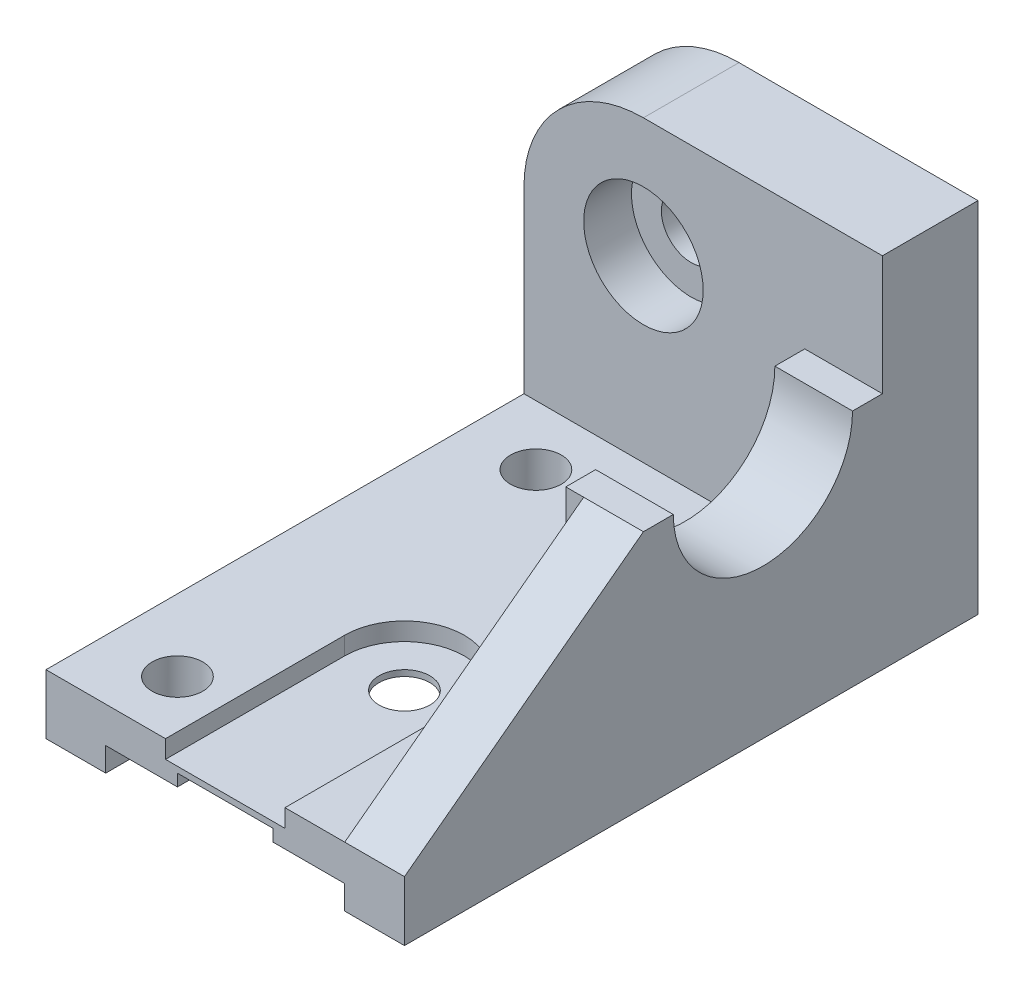
ISO-10303-21;
HEADER;
FILE_DESCRIPTION(('STEP AP214'),'2;1');
FILE_NAME('part.step','',(''),(''),'','','');
FILE_SCHEMA(('AUTOMOTIVE_DESIGN { 1 0 10303 214 1 1 1 1 }'));
ENDSEC;
DATA;
#1=APPLICATION_CONTEXT('core data for automotive mechanical design processes');
#2=APPLICATION_PROTOCOL_DEFINITION('international standard','automotive_design',2000,#1);
#3=PRODUCT_CONTEXT('',#1,'mechanical');
#4=PRODUCT('Part','Part','',(#3));
#5=PRODUCT_RELATED_PRODUCT_CATEGORY('part','',(#4));
#6=PRODUCT_DEFINITION_FORMATION('','',#4);
#7=PRODUCT_DEFINITION_CONTEXT('part definition',#1,'design');
#8=PRODUCT_DEFINITION('design','',#6,#7);
#9=PRODUCT_DEFINITION_SHAPE('','',#8);
#10=(LENGTH_UNIT() NAMED_UNIT(*) SI_UNIT(.MILLI.,.METRE.));
#11=(NAMED_UNIT(*) PLANE_ANGLE_UNIT() SI_UNIT($,.RADIAN.));
#12=(NAMED_UNIT(*) SI_UNIT($,.STERADIAN.) SOLID_ANGLE_UNIT());
#13=UNCERTAINTY_MEASURE_WITH_UNIT(LENGTH_MEASURE(1.E-05),#10,'distance_accuracy_value','');
#14=(GEOMETRIC_REPRESENTATION_CONTEXT(3) GLOBAL_UNCERTAINTY_ASSIGNED_CONTEXT((#13)) GLOBAL_UNIT_ASSIGNED_CONTEXT((#10,
#11,#12)) REPRESENTATION_CONTEXT('',''));
#15=CARTESIAN_POINT('',(0.,0.,0.));
#16=DIRECTION('',(0.,0.,1.));
#17=DIRECTION('',(1.,0.,0.));
#18=AXIS2_PLACEMENT_3D('',#15,#16,#17);
#19=CARTESIAN_POINT('',(600.,400.,-400.));
#20=DIRECTION('',(0.,-1.,0.));
#21=DIRECTION('',(0.,0.,-1.));
#22=AXIS2_PLACEMENT_3D('',#19,#20,#21);
#23=PLANE('',#22);
#24=DIRECTION('',(0.,0.,-1.));
#25=VECTOR('',#24,1.);
#26=CARTESIAN_POINT('',(470.,400.,-400.));
#27=LINE('',#26,#25);
#28=CARTESIAN_POINT('',(470.,400.,-750.));
#29=VERTEX_POINT('',#28);
#30=CARTESIAN_POINT('',(470.,400.,-800.));
#31=VERTEX_POINT('',#30);
#32=EDGE_CURVE('E288',#29,#31,#27,.T.);
#33=ORIENTED_EDGE('',*,*,#32,.F.);
#34=DIRECTION('',(1.,0.,0.));
#35=VECTOR('',#34,1.);
#36=CARTESIAN_POINT('',(200.,400.,-750.));
#37=LINE('',#36,#35);
#38=CARTESIAN_POINT('',(600.,400.,-750.));
#39=VERTEX_POINT('',#38);
#40=EDGE_CURVE('E271',#29,#39,#37,.T.);
#41=ORIENTED_EDGE('',*,*,#40,.T.);
#42=DIRECTION('',(0.,0.,-1.));
#43=VECTOR('',#42,1.);
#44=CARTESIAN_POINT('',(600.,400.,-400.));
#45=LINE('',#44,#43);
#46=CARTESIAN_POINT('',(600.,400.,-800.));
#47=VERTEX_POINT('',#46);
#48=EDGE_CURVE('E250',#39,#47,#45,.T.);
#49=ORIENTED_EDGE('',*,*,#48,.T.);
#50=DIRECTION('',(-1.,0.,0.));
#51=VECTOR('',#50,1.);
#52=CARTESIAN_POINT('',(600.,400.,-800.));
#53=LINE('',#52,#51);
#54=EDGE_CURVE('E273',#47,#31,#53,.T.);
#55=ORIENTED_EDGE('',*,*,#54,.T.);
#56=EDGE_LOOP('',(#33,#41,#49,#55));
#57=FACE_BOUND('',#56,.T.);
#58=ADVANCED_FACE('F44',(#57),#23,.F.);
#59=CARTESIAN_POINT('',(600.,100.,-960.));
#60=DIRECTION('',(0.,1.,0.));
#61=DIRECTION('',(0.,0.,1.));
#62=AXIS2_PLACEMENT_3D('',#59,#60,#61);
#63=PLANE('',#62);
#64=DIRECTION('',(0.,0.,-1.));
#65=VECTOR('',#64,1.);
#66=CARTESIAN_POINT('',(500.,100.,-400.));
#67=LINE('',#66,#65);
#68=CARTESIAN_POINT('',(500.,100.,0.));
#69=VERTEX_POINT('',#68);
#70=CARTESIAN_POINT('',(500.,100.,-400.));
#71=VERTEX_POINT('',#70);
#72=EDGE_CURVE('E63',#69,#71,#67,.T.);
#73=ORIENTED_EDGE('',*,*,#72,.T.);
#74=DIRECTION('',(1.,0.,0.));
#75=VECTOR('',#74,1.);
#76=CARTESIAN_POINT('',(600.,100.,-400.));
#77=LINE('',#76,#75);
#78=CARTESIAN_POINT('',(470.,100.,-400.));
#79=VERTEX_POINT('',#78);
#80=EDGE_CURVE('E276',#79,#71,#77,.T.);
#81=ORIENTED_EDGE('',*,*,#80,.F.);
#82=DIRECTION('',(0.,0.,-1.));
#83=VECTOR('',#82,1.);
#84=CARTESIAN_POINT('',(470.,100.,-400.));
#85=LINE('',#84,#83);
#86=CARTESIAN_POINT('',(470.,100.,-800.));
#87=VERTEX_POINT('',#86);
#88=EDGE_CURVE('E281',#79,#87,#85,.T.);
#89=ORIENTED_EDGE('',*,*,#88,.T.);
#90=DIRECTION('',(1.,0.,0.));
#91=VECTOR('',#90,1.);
#92=CARTESIAN_POINT('',(0.,100.,-800.));
#93=LINE('',#92,#91);
#94=CARTESIAN_POINT('',(0.,100.,-800.));
#95=VERTEX_POINT('',#94);
#96=EDGE_CURVE('E359',#95,#87,#93,.T.);
#97=ORIENTED_EDGE('',*,*,#96,.F.);
#98=DIRECTION('',(0.,0.,1.));
#99=VECTOR('',#98,1.);
#100=CARTESIAN_POINT('',(0.,100.,-960.));
#101=LINE('',#100,#99);
#102=CARTESIAN_POINT('',(0.,100.,0.));
#103=VERTEX_POINT('',#102);
#104=EDGE_CURVE('E442',#95,#103,#101,.T.);
#105=ORIENTED_EDGE('',*,*,#104,.T.);
#106=DIRECTION('',(-1.,0.,0.));
#107=VECTOR('',#106,1.);
#108=CARTESIAN_POINT('',(600.,100.,0.));
#109=LINE('',#108,#107);
#110=CARTESIAN_POINT('',(200.,100.,0.));
#111=VERTEX_POINT('',#110);
#112=EDGE_CURVE('E441',#111,#103,#109,.T.);
#113=ORIENTED_EDGE('',*,*,#112,.F.);
#114=DIRECTION('',(0.,0.,1.));
#115=VECTOR('',#114,1.);
#116=CARTESIAN_POINT('',(200.,100.,-300.));
#117=LINE('',#116,#115);
#118=CARTESIAN_POINT('',(200.,100.,-300.));
#119=VERTEX_POINT('',#118);
#120=EDGE_CURVE('E312',#119,#111,#117,.T.);
#121=ORIENTED_EDGE('',*,*,#120,.F.);
#122=CARTESIAN_POINT('',(300.,100.,-300.));
#123=DIRECTION('',(0.,1.,0.));
#124=DIRECTION('',(0.,0.,1.));
#125=AXIS2_PLACEMENT_3D('',#122,#123,#124);
#126=CIRCLE('',#125,99.9999999999999);
#127=CARTESIAN_POINT('',(400.,100.,-300.));
#128=VERTEX_POINT('',#127);
#129=EDGE_CURVE('E296',#128,#119,#126,.T.);
#130=ORIENTED_EDGE('',*,*,#129,.F.);
#131=DIRECTION('',(0.,0.,-1.));
#132=VECTOR('',#131,1.);
#133=CARTESIAN_POINT('',(400.,100.,0.));
#134=LINE('',#133,#132);
#135=CARTESIAN_POINT('',(400.,100.,0.));
#136=VERTEX_POINT('',#135);
#137=EDGE_CURVE('E303',#136,#128,#134,.T.);
#138=ORIENTED_EDGE('',*,*,#137,.F.);
#139=EDGE_CURVE('E58',#69,#136,#109,.T.);
#140=ORIENTED_EDGE('',*,*,#139,.F.);
#141=EDGE_LOOP('',(#73,#81,#89,#97,#105,#113,#121,#130,#138,#140));
#142=FACE_BOUND('',#141,.T.);
#143=CARTESIAN_POINT('',(120.,100.,-700.));
#144=DIRECTION('',(0.,1.,0.));
#145=DIRECTION('',(0.,0.,1.));
#146=AXIS2_PLACEMENT_3D('',#143,#144,#145);
#147=CIRCLE('',#146,42.5);
#148=CARTESIAN_POINT('',(120.,100.,-657.5));
#149=VERTEX_POINT('',#148);
#150=EDGE_CURVE('E334',#149,#149,#147,.T.);
#151=ORIENTED_EDGE('',*,*,#150,.F.);
#152=EDGE_LOOP('',(#151));
#153=FACE_BOUND('',#152,.T.);
#154=CARTESIAN_POINT('',(120.,100.,-100.));
#155=DIRECTION('',(0.,1.,0.));
#156=DIRECTION('',(0.,0.,1.));
#157=AXIS2_PLACEMENT_3D('',#154,#155,#156);
#158=CIRCLE('',#157,42.5);
#159=CARTESIAN_POINT('',(120.,100.,-57.5));
#160=VERTEX_POINT('',#159);
#161=EDGE_CURVE('E316',#160,#160,#158,.T.);
#162=ORIENTED_EDGE('',*,*,#161,.F.);
#163=EDGE_LOOP('',(#162));
#164=FACE_BOUND('',#163,.T.);
#165=ADVANCED_FACE('F505',(#142,#153,#164),#63,.T.);
#166=CARTESIAN_POINT('',(0.,600.,-800.));
#167=DIRECTION('',(0.,0.,-1.));
#168=DIRECTION('',(-1.,0.,0.));
#169=AXIS2_PLACEMENT_3D('',#166,#167,#168);
#170=PLANE('',#169);
#171=CARTESIAN_POINT('',(200.,400.,-800.));
#172=DIRECTION('',(0.,0.,1.));
#173=DIRECTION('',(1.,0.,0.));
#174=AXIS2_PLACEMENT_3D('',#171,#172,#173);
#175=CIRCLE('',#174,100.);
#176=CARTESIAN_POINT('',(300.,400.,-800.));
#177=VERTEX_POINT('',#176);
#178=EDGE_CURVE('E353',#177,#177,#175,.T.);
#179=ORIENTED_EDGE('',*,*,#178,.F.);
#180=EDGE_LOOP('',(#179));
#181=FACE_BOUND('',#180,.T.);
#182=ORIENTED_EDGE('',*,*,#54,.F.);
#183=DIRECTION('',(0.,-1.,0.));
#184=VECTOR('',#183,1.);
#185=CARTESIAN_POINT('',(600.,600.,-800.));
#186=LINE('',#185,#184);
#187=CARTESIAN_POINT('',(600.,600.,-800.));
#188=VERTEX_POINT('',#187);
#189=EDGE_CURVE('E371',#188,#47,#186,.T.);
#190=ORIENTED_EDGE('',*,*,#189,.F.);
#191=DIRECTION('',(1.,0.,0.));
#192=VECTOR('',#191,1.);
#193=CARTESIAN_POINT('',(0.,600.,-800.));
#194=LINE('',#193,#192);
#195=CARTESIAN_POINT('',(200.,600.,-800.));
#196=VERTEX_POINT('',#195);
#197=EDGE_CURVE('E361',#196,#188,#194,.T.);
#198=ORIENTED_EDGE('',*,*,#197,.F.);
#199=CARTESIAN_POINT('',(200.,400.,-800.));
#200=DIRECTION('',(0.,0.,-1.));
#201=DIRECTION('',(-1.,0.,0.));
#202=AXIS2_PLACEMENT_3D('',#199,#200,#201);
#203=CIRCLE('',#202,200.);
#204=CARTESIAN_POINT('',(0.,400.,-800.));
#205=VERTEX_POINT('',#204);
#206=EDGE_CURVE('E471',#196,#205,#203,.F.);
#207=ORIENTED_EDGE('',*,*,#206,.T.);
#208=DIRECTION('',(0.,-1.,0.));
#209=VECTOR('',#208,1.);
#210=CARTESIAN_POINT('',(0.,600.,-800.));
#211=LINE('',#210,#209);
#212=EDGE_CURVE('E374',#205,#95,#211,.T.);
#213=ORIENTED_EDGE('',*,*,#212,.T.);
#214=ORIENTED_EDGE('',*,*,#96,.T.);
#215=DIRECTION('',(0.,-1.,0.));
#216=VECTOR('',#215,1.);
#217=CARTESIAN_POINT('',(470.,100.,-800.));
#218=LINE('',#217,#216);
#219=EDGE_CURVE('E282',#31,#87,#218,.T.);
#220=ORIENTED_EDGE('',*,*,#219,.F.);
#221=EDGE_LOOP('',(#182,#190,#198,#207,#213,#214,#220));
#222=FACE_BOUND('',#221,.T.);
#223=ADVANCED_FACE('F494',(#181,#222),#170,.F.);
#224=CARTESIAN_POINT('',(100.,0.,-960.));
#225=DIRECTION('',(1.,0.,0.));
#226=DIRECTION('',(0.,0.,-1.));
#227=AXIS2_PLACEMENT_3D('',#224,#225,#226);
#228=PLANE('',#227);
#229=DIRECTION('',(0.,1.,0.));
#230=VECTOR('',#229,1.);
#231=CARTESIAN_POINT('',(100.,0.,-737.5));
#232=LINE('',#231,#230);
#233=CARTESIAN_POINT('',(100.,0.,-737.5));
#234=VERTEX_POINT('',#233);
#235=CARTESIAN_POINT('',(100.,40.,-737.5));
#236=VERTEX_POINT('',#235);
#237=EDGE_CURVE('E348',#234,#236,#232,.T.);
#238=ORIENTED_EDGE('',*,*,#237,.F.);
#239=DIRECTION('',(0.,0.,1.));
#240=VECTOR('',#239,1.);
#241=CARTESIAN_POINT('',(100.,0.,-960.));
#242=LINE('',#241,#240);
#243=CARTESIAN_POINT('',(100.,0.,-960.));
#244=VERTEX_POINT('',#243);
#245=EDGE_CURVE('E467',#244,#234,#242,.T.);
#246=ORIENTED_EDGE('',*,*,#245,.F.);
#247=DIRECTION('',(0.,1.,0.));
#248=VECTOR('',#247,1.);
#249=CARTESIAN_POINT('',(100.,0.,-960.));
#250=LINE('',#249,#248);
#251=CARTESIAN_POINT('',(100.,40.,-960.));
#252=VERTEX_POINT('',#251);
#253=EDGE_CURVE('E384',#244,#252,#250,.T.);
#254=ORIENTED_EDGE('',*,*,#253,.T.);
#255=DIRECTION('',(0.,0.,1.));
#256=VECTOR('',#255,1.);
#257=CARTESIAN_POINT('',(100.,40.,-960.));
#258=LINE('',#257,#256);
#259=EDGE_CURVE('E464',#252,#236,#258,.T.);
#260=ORIENTED_EDGE('',*,*,#259,.T.);
#261=EDGE_LOOP('',(#238,#246,#254,#260));
#262=FACE_BOUND('',#261,.T.);
#263=ADVANCED_FACE('F543',(#262),#228,.T.);
#264=DIRECTION('',(0.,1.,0.));
#265=VECTOR('',#264,1.);
#266=CARTESIAN_POINT('',(100.,0.,-662.5));
#267=LINE('',#266,#265);
#268=CARTESIAN_POINT('',(100.,40.,-662.5));
#269=VERTEX_POINT('',#268);
#270=CARTESIAN_POINT('',(100.,0.,-662.5));
#271=VERTEX_POINT('',#270);
#272=EDGE_CURVE('E341',#269,#271,#267,.F.);
#273=ORIENTED_EDGE('',*,*,#272,.F.);
#274=CARTESIAN_POINT('',(100.,40.,-137.5));
#275=VERTEX_POINT('',#274);
#276=EDGE_CURVE('E463',#269,#275,#258,.T.);
#277=ORIENTED_EDGE('',*,*,#276,.T.);
#278=DIRECTION('',(0.,1.,0.));
#279=VECTOR('',#278,1.);
#280=CARTESIAN_POINT('',(100.,0.,-137.5));
#281=LINE('',#280,#279);
#282=CARTESIAN_POINT('',(100.,0.,-137.5));
#283=VERTEX_POINT('',#282);
#284=EDGE_CURVE('E345',#283,#275,#281,.T.);
#285=ORIENTED_EDGE('',*,*,#284,.F.);
#286=EDGE_CURVE('E469',#271,#283,#242,.T.);
#287=ORIENTED_EDGE('',*,*,#286,.F.);
#288=EDGE_LOOP('',(#273,#277,#285,#287));
#289=FACE_BOUND('',#288,.T.);
#290=ADVANCED_FACE('F623',(#289),#228,.T.);
#291=CARTESIAN_POINT('',(0.,100.,-960.));
#292=DIRECTION('',(-1.,0.,0.));
#293=DIRECTION('',(0.,0.,1.));
#294=AXIS2_PLACEMENT_3D('',#291,#292,#293);
#295=PLANE('',#294);
#296=ORIENTED_EDGE('',*,*,#212,.F.);
#297=DIRECTION('',(0.,0.,1.));
#298=VECTOR('',#297,1.);
#299=CARTESIAN_POINT('',(0.,400.,-960.));
#300=LINE('',#299,#298);
#301=CARTESIAN_POINT('',(0.,400.,-960.));
#302=VERTEX_POINT('',#301);
#303=EDGE_CURVE('E476',#205,#302,#300,.F.);
#304=ORIENTED_EDGE('',*,*,#303,.T.);
#305=DIRECTION('',(0.,-1.,0.));
#306=VECTOR('',#305,1.);
#307=CARTESIAN_POINT('',(0.,100.,-960.));
#308=LINE('',#307,#306);
#309=CARTESIAN_POINT('',(0.,0.,-960.));
#310=VERTEX_POINT('',#309);
#311=EDGE_CURVE('E377',#302,#310,#308,.T.);
#312=ORIENTED_EDGE('',*,*,#311,.T.);
#313=DIRECTION('',(0.,0.,1.));
#314=VECTOR('',#313,1.);
#315=CARTESIAN_POINT('',(0.,0.,-960.));
#316=LINE('',#315,#314);
#317=CARTESIAN_POINT('',(0.,0.,0.));
#318=VERTEX_POINT('',#317);
#319=EDGE_CURVE('E406',#310,#318,#316,.T.);
#320=ORIENTED_EDGE('',*,*,#319,.T.);
#321=DIRECTION('',(0.,-1.,0.));
#322=VECTOR('',#321,1.);
#323=CARTESIAN_POINT('',(0.,100.,0.));
#324=LINE('',#323,#322);
#325=EDGE_CURVE('E380',#103,#318,#324,.T.);
#326=ORIENTED_EDGE('',*,*,#325,.F.);
#327=ORIENTED_EDGE('',*,*,#104,.F.);
#328=EDGE_LOOP('',(#296,#304,#312,#320,#326,#327));
#329=FACE_BOUND('',#328,.T.);
#330=ADVANCED_FACE('F497',(#329),#295,.T.);
#331=CARTESIAN_POINT('',(600.,0.,-960.));
#332=DIRECTION('',(1.,0.,0.));
#333=DIRECTION('',(0.,0.,-1.));
#334=AXIS2_PLACEMENT_3D('',#331,#332,#333);
#335=PLANE('',#334);
#336=DIRECTION('',(0.,-0.6,0.8));
#337=VECTOR('',#336,1.);
#338=CARTESIAN_POINT('',(600.,100.,0.));
#339=LINE('',#338,#337);
#340=CARTESIAN_POINT('',(600.,400.,-400.));
#341=VERTEX_POINT('',#340);
#342=CARTESIAN_POINT('',(600.,100.,0.));
#343=VERTEX_POINT('',#342);
#344=EDGE_CURVE('E241',#341,#343,#339,.T.);
#345=ORIENTED_EDGE('',*,*,#344,.T.);
#346=DIRECTION('',(0.,1.,0.));
#347=VECTOR('',#346,1.);
#348=CARTESIAN_POINT('',(600.,0.,0.));
#349=LINE('',#348,#347);
#350=CARTESIAN_POINT('',(600.,0.,0.));
#351=VERTEX_POINT('',#350);
#352=EDGE_CURVE('E437',#351,#343,#349,.T.);
#353=ORIENTED_EDGE('',*,*,#352,.F.);
#354=DIRECTION('',(0.,0.,1.));
#355=VECTOR('',#354,1.);
#356=CARTESIAN_POINT('',(600.,0.,-960.));
#357=LINE('',#356,#355);
#358=CARTESIAN_POINT('',(600.,0.,-960.));
#359=VERTEX_POINT('',#358);
#360=EDGE_CURVE('E450',#359,#351,#357,.T.);
#361=ORIENTED_EDGE('',*,*,#360,.F.);
#362=DIRECTION('',(0.,1.,0.));
#363=VECTOR('',#362,1.);
#364=CARTESIAN_POINT('',(600.,0.,-960.));
#365=LINE('',#364,#363);
#366=CARTESIAN_POINT('',(600.,600.,-960.));
#367=VERTEX_POINT('',#366);
#368=EDGE_CURVE('E410',#359,#367,#365,.T.);
#369=ORIENTED_EDGE('',*,*,#368,.T.);
#370=DIRECTION('',(0.,0.,-1.));
#371=VECTOR('',#370,1.);
#372=CARTESIAN_POINT('',(600.,600.,-960.));
#373=LINE('',#372,#371);
#374=EDGE_CURVE('E362',#188,#367,#373,.T.);
#375=ORIENTED_EDGE('',*,*,#374,.F.);
#376=ORIENTED_EDGE('',*,*,#189,.T.);
#377=ORIENTED_EDGE('',*,*,#48,.F.);
#378=CARTESIAN_POINT('',(600.,400.,-600.));
#379=DIRECTION('',(1.,0.,0.));
#380=DIRECTION('',(0.,0.,-1.));
#381=AXIS2_PLACEMENT_3D('',#378,#379,#380);
#382=CIRCLE('',#381,150.);
#383=CARTESIAN_POINT('',(600.,400.,-450.));
#384=VERTEX_POINT('',#383);
#385=EDGE_CURVE('E243',#384,#39,#382,.T.);
#386=ORIENTED_EDGE('',*,*,#385,.F.);
#387=EDGE_CURVE('E236',#341,#384,#45,.T.);
#388=ORIENTED_EDGE('',*,*,#387,.F.);
#389=EDGE_LOOP('',(#345,#353,#361,#369,#375,#376,#377,#386,#388));
#390=FACE_BOUND('',#389,.T.);
#391=ADVANCED_FACE('F238',(#390),#335,.T.);
#392=CARTESIAN_POINT('',(500.,0.,-960.));
#393=DIRECTION('',(0.,-1.,0.));
#394=DIRECTION('',(0.,0.,-1.));
#395=AXIS2_PLACEMENT_3D('',#392,#393,#394);
#396=PLANE('',#395);
#397=DIRECTION('',(1.,0.,0.));
#398=VECTOR('',#397,1.);
#399=CARTESIAN_POINT('',(500.,0.,0.));
#400=LINE('',#399,#398);
#401=CARTESIAN_POINT('',(500.,0.,0.));
#402=VERTEX_POINT('',#401);
#403=EDGE_CURVE('E436',#402,#351,#400,.T.);
#404=ORIENTED_EDGE('',*,*,#403,.F.);
#405=DIRECTION('',(0.,0.,1.));
#406=VECTOR('',#405,1.);
#407=CARTESIAN_POINT('',(500.,0.,-960.));
#408=LINE('',#407,#406);
#409=CARTESIAN_POINT('',(500.,0.,-960.));
#410=VERTEX_POINT('',#409);
#411=EDGE_CURVE('E446',#410,#402,#408,.T.);
#412=ORIENTED_EDGE('',*,*,#411,.F.);
#413=DIRECTION('',(1.,0.,0.));
#414=VECTOR('',#413,1.);
#415=CARTESIAN_POINT('',(500.,0.,-960.));
#416=LINE('',#415,#414);
#417=EDGE_CURVE('E404',#410,#359,#416,.T.);
#418=ORIENTED_EDGE('',*,*,#417,.T.);
#419=ORIENTED_EDGE('',*,*,#360,.T.);
#420=EDGE_LOOP('',(#404,#412,#418,#419));
#421=FACE_BOUND('',#420,.T.);
#422=ADVANCED_FACE('F511',(#421),#396,.T.);
#423=CARTESIAN_POINT('',(500.,40.,-960.));
#424=DIRECTION('',(-1.,0.,0.));
#425=DIRECTION('',(0.,0.,1.));
#426=AXIS2_PLACEMENT_3D('',#423,#424,#425);
#427=PLANE('',#426);
#428=DIRECTION('',(0.,-1.,0.));
#429=VECTOR('',#428,1.);
#430=CARTESIAN_POINT('',(500.,40.,0.));
#431=LINE('',#430,#429);
#432=CARTESIAN_POINT('',(500.,40.,0.));
#433=VERTEX_POINT('',#432);
#434=EDGE_CURVE('E433',#433,#402,#431,.T.);
#435=ORIENTED_EDGE('',*,*,#434,.F.);
#436=DIRECTION('',(0.,0.,1.));
#437=VECTOR('',#436,1.);
#438=CARTESIAN_POINT('',(500.,40.,-960.));
#439=LINE('',#438,#437);
#440=CARTESIAN_POINT('',(500.,40.,-960.));
#441=VERTEX_POINT('',#440);
#442=EDGE_CURVE('E452',#441,#433,#439,.T.);
#443=ORIENTED_EDGE('',*,*,#442,.F.);
#444=DIRECTION('',(0.,-1.,0.));
#445=VECTOR('',#444,1.);
#446=CARTESIAN_POINT('',(500.,40.,-960.));
#447=LINE('',#446,#445);
#448=EDGE_CURVE('E402',#441,#410,#447,.T.);
#449=ORIENTED_EDGE('',*,*,#448,.T.);
#450=ORIENTED_EDGE('',*,*,#411,.T.);
#451=EDGE_LOOP('',(#435,#443,#449,#450));
#452=FACE_BOUND('',#451,.T.);
#453=ADVANCED_FACE('F520',(#452),#427,.T.);
#454=CARTESIAN_POINT('',(380.,40.,-960.));
#455=DIRECTION('',(0.,-1.,0.));
#456=DIRECTION('',(0.,0.,-1.));
#457=AXIS2_PLACEMENT_3D('',#454,#455,#456);
#458=PLANE('',#457);
#459=DIRECTION('',(1.,0.,0.));
#460=VECTOR('',#459,1.);
#461=CARTESIAN_POINT('',(380.,40.,0.));
#462=LINE('',#461,#460);
#463=CARTESIAN_POINT('',(380.,40.,0.));
#464=VERTEX_POINT('',#463);
#465=EDGE_CURVE('E427',#464,#433,#462,.T.);
#466=ORIENTED_EDGE('',*,*,#465,.F.);
#467=DIRECTION('',(0.,0.,1.));
#468=VECTOR('',#467,1.);
#469=CARTESIAN_POINT('',(380.,40.,-960.));
#470=LINE('',#469,#468);
#471=CARTESIAN_POINT('',(380.,40.,-960.));
#472=VERTEX_POINT('',#471);
#473=EDGE_CURVE('E454',#472,#464,#470,.T.);
#474=ORIENTED_EDGE('',*,*,#473,.F.);
#475=DIRECTION('',(1.,0.,0.));
#476=VECTOR('',#475,1.);
#477=CARTESIAN_POINT('',(380.,40.,-960.));
#478=LINE('',#477,#476);
#479=EDGE_CURVE('E400',#472,#441,#478,.T.);
#480=ORIENTED_EDGE('',*,*,#479,.T.);
#481=ORIENTED_EDGE('',*,*,#442,.T.);
#482=EDGE_LOOP('',(#466,#474,#480,#481));
#483=FACE_BOUND('',#482,.T.);
#484=ADVANCED_FACE('F525',(#483),#458,.T.);
#485=CARTESIAN_POINT('',(380.,60.,-960.));
#486=DIRECTION('',(-1.,0.,0.));
#487=DIRECTION('',(0.,0.,1.));
#488=AXIS2_PLACEMENT_3D('',#485,#486,#487);
#489=PLANE('',#488);
#490=DIRECTION('',(0.,-1.,0.));
#491=VECTOR('',#490,1.);
#492=CARTESIAN_POINT('',(380.,60.,0.));
#493=LINE('',#492,#491);
#494=CARTESIAN_POINT('',(380.,60.,0.));
#495=VERTEX_POINT('',#494);
#496=EDGE_CURVE('E430',#495,#464,#493,.T.);
#497=ORIENTED_EDGE('',*,*,#496,.F.);
#498=DIRECTION('',(0.,0.,1.));
#499=VECTOR('',#498,1.);
#500=CARTESIAN_POINT('',(380.,60.,-960.));
#501=LINE('',#500,#499);
#502=CARTESIAN_POINT('',(380.,60.,-960.));
#503=VERTEX_POINT('',#502);
#504=EDGE_CURVE('E453',#503,#495,#501,.T.);
#505=ORIENTED_EDGE('',*,*,#504,.F.);
#506=DIRECTION('',(0.,-1.,0.));
#507=VECTOR('',#506,1.);
#508=CARTESIAN_POINT('',(380.,60.,-960.));
#509=LINE('',#508,#507);
#510=EDGE_CURVE('E394',#503,#472,#509,.T.);
#511=ORIENTED_EDGE('',*,*,#510,.T.);
#512=ORIENTED_EDGE('',*,*,#473,.T.);
#513=EDGE_LOOP('',(#497,#505,#511,#512));
#514=FACE_BOUND('',#513,.T.);
#515=ADVANCED_FACE('F524',(#514),#489,.T.);
#516=CARTESIAN_POINT('',(220.,60.,-960.));
#517=DIRECTION('',(0.,-1.,0.));
#518=DIRECTION('',(0.,0.,-1.));
#519=AXIS2_PLACEMENT_3D('',#516,#517,#518);
#520=PLANE('',#519);
#521=CARTESIAN_POINT('',(300.,60.,-300.));
#522=DIRECTION('',(0.,-1.,0.));
#523=DIRECTION('',(0.,0.,-1.));
#524=AXIS2_PLACEMENT_3D('',#521,#522,#523);
#525=CIRCLE('',#524,42.5);
#526=CARTESIAN_POINT('',(300.,60.,-342.5));
#527=VERTEX_POINT('',#526);
#528=EDGE_CURVE('E294',#527,#527,#525,.T.);
#529=ORIENTED_EDGE('',*,*,#528,.F.);
#530=EDGE_LOOP('',(#529));
#531=FACE_BOUND('',#530,.T.);
#532=DIRECTION('',(1.,0.,0.));
#533=VECTOR('',#532,1.);
#534=CARTESIAN_POINT('',(220.,60.,0.));
#535=LINE('',#534,#533);
#536=CARTESIAN_POINT('',(220.,60.,0.));
#537=VERTEX_POINT('',#536);
#538=EDGE_CURVE('E425',#537,#495,#535,.T.);
#539=ORIENTED_EDGE('',*,*,#538,.F.);
#540=DIRECTION('',(0.,0.,1.));
#541=VECTOR('',#540,1.);
#542=CARTESIAN_POINT('',(220.,60.,-960.));
#543=LINE('',#542,#541);
#544=CARTESIAN_POINT('',(220.,60.,-960.));
#545=VERTEX_POINT('',#544);
#546=EDGE_CURVE('E460',#545,#537,#543,.T.);
#547=ORIENTED_EDGE('',*,*,#546,.F.);
#548=DIRECTION('',(1.,0.,0.));
#549=VECTOR('',#548,1.);
#550=CARTESIAN_POINT('',(220.,60.,-960.));
#551=LINE('',#550,#549);
#552=EDGE_CURVE('E395',#545,#503,#551,.T.);
#553=ORIENTED_EDGE('',*,*,#552,.T.);
#554=ORIENTED_EDGE('',*,*,#504,.T.);
#555=EDGE_LOOP('',(#539,#547,#553,#554));
#556=FACE_BOUND('',#555,.T.);
#557=ADVANCED_FACE('F527',(#531,#556),#520,.T.);
#558=CARTESIAN_POINT('',(220.,40.,-960.));
#559=DIRECTION('',(1.,0.,0.));
#560=DIRECTION('',(0.,0.,-1.));
#561=AXIS2_PLACEMENT_3D('',#558,#559,#560);
#562=PLANE('',#561);
#563=DIRECTION('',(0.,1.,0.));
#564=VECTOR('',#563,1.);
#565=CARTESIAN_POINT('',(220.,40.,0.));
#566=LINE('',#565,#564);
#567=CARTESIAN_POINT('',(220.,40.,0.));
#568=VERTEX_POINT('',#567);
#569=EDGE_CURVE('E423',#568,#537,#566,.T.);
#570=ORIENTED_EDGE('',*,*,#569,.F.);
#571=DIRECTION('',(0.,0.,1.));
#572=VECTOR('',#571,1.);
#573=CARTESIAN_POINT('',(220.,40.,-960.));
#574=LINE('',#573,#572);
#575=CARTESIAN_POINT('',(220.,40.,-960.));
#576=VERTEX_POINT('',#575);
#577=EDGE_CURVE('E457',#576,#568,#574,.T.);
#578=ORIENTED_EDGE('',*,*,#577,.F.);
#579=DIRECTION('',(0.,1.,0.));
#580=VECTOR('',#579,1.);
#581=CARTESIAN_POINT('',(220.,40.,-960.));
#582=LINE('',#581,#580);
#583=EDGE_CURVE('E386',#576,#545,#582,.T.);
#584=ORIENTED_EDGE('',*,*,#583,.T.);
#585=ORIENTED_EDGE('',*,*,#546,.T.);
#586=EDGE_LOOP('',(#570,#578,#584,#585));
#587=FACE_BOUND('',#586,.T.);
#588=ADVANCED_FACE('F531',(#587),#562,.T.);
#589=CARTESIAN_POINT('',(100.,40.,-960.));
#590=DIRECTION('',(0.,-1.,0.));
#591=DIRECTION('',(0.,0.,-1.));
#592=AXIS2_PLACEMENT_3D('',#589,#590,#591);
#593=PLANE('',#592);
#594=CARTESIAN_POINT('',(120.,40.,-700.));
#595=DIRECTION('',(0.,-1.,0.));
#596=DIRECTION('',(0.,0.,-1.));
#597=AXIS2_PLACEMENT_3D('',#594,#595,#596);
#598=CIRCLE('',#597,42.5);
#599=EDGE_CURVE('E346',#236,#269,#598,.T.);
#600=ORIENTED_EDGE('',*,*,#599,.F.);
#601=ORIENTED_EDGE('',*,*,#259,.F.);
#602=DIRECTION('',(1.,0.,0.));
#603=VECTOR('',#602,1.);
#604=CARTESIAN_POINT('',(100.,40.,-960.));
#605=LINE('',#604,#603);
#606=EDGE_CURVE('E387',#252,#576,#605,.T.);
#607=ORIENTED_EDGE('',*,*,#606,.T.);
#608=ORIENTED_EDGE('',*,*,#577,.T.);
#609=DIRECTION('',(1.,0.,0.));
#610=VECTOR('',#609,1.);
#611=CARTESIAN_POINT('',(100.,40.,0.));
#612=LINE('',#611,#610);
#613=CARTESIAN_POINT('',(100.,40.,0.));
#614=VERTEX_POINT('',#613);
#615=EDGE_CURVE('E420',#614,#568,#612,.T.);
#616=ORIENTED_EDGE('',*,*,#615,.F.);
#617=CARTESIAN_POINT('',(100.,40.,-62.5));
#618=VERTEX_POINT('',#617);
#619=EDGE_CURVE('E462',#618,#614,#258,.T.);
#620=ORIENTED_EDGE('',*,*,#619,.F.);
#621=CARTESIAN_POINT('',(120.,40.,-100.));
#622=DIRECTION('',(0.,-1.,0.));
#623=DIRECTION('',(0.,0.,-1.));
#624=AXIS2_PLACEMENT_3D('',#621,#622,#623);
#625=CIRCLE('',#624,42.5);
#626=EDGE_CURVE('E338',#275,#618,#625,.T.);
#627=ORIENTED_EDGE('',*,*,#626,.F.);
#628=ORIENTED_EDGE('',*,*,#276,.F.);
#629=EDGE_LOOP('',(#600,#601,#607,#608,#616,#620,#627,#628));
#630=FACE_BOUND('',#629,.T.);
#631=ADVANCED_FACE('F539',(#630),#593,.T.);
#632=DIRECTION('',(0.,1.,0.));
#633=VECTOR('',#632,1.);
#634=CARTESIAN_POINT('',(100.,0.,-62.5));
#635=LINE('',#634,#633);
#636=CARTESIAN_POINT('',(100.,0.,-62.5));
#637=VERTEX_POINT('',#636);
#638=EDGE_CURVE('E329',#618,#637,#635,.F.);
#639=ORIENTED_EDGE('',*,*,#638,.F.);
#640=ORIENTED_EDGE('',*,*,#619,.T.);
#641=DIRECTION('',(0.,1.,0.));
#642=VECTOR('',#641,1.);
#643=CARTESIAN_POINT('',(100.,0.,0.));
#644=LINE('',#643,#642);
#645=CARTESIAN_POINT('',(100.,0.,0.));
#646=VERTEX_POINT('',#645);
#647=EDGE_CURVE('E414',#646,#614,#644,.T.);
#648=ORIENTED_EDGE('',*,*,#647,.F.);
#649=EDGE_CURVE('E468',#637,#646,#242,.T.);
#650=ORIENTED_EDGE('',*,*,#649,.F.);
#651=EDGE_LOOP('',(#639,#640,#648,#650));
#652=FACE_BOUND('',#651,.T.);
#653=ADVANCED_FACE('F617',(#652),#228,.T.);
#654=CARTESIAN_POINT('',(0.,0.,-960.));
#655=DIRECTION('',(0.,-1.,0.));
#656=DIRECTION('',(0.,0.,-1.));
#657=AXIS2_PLACEMENT_3D('',#654,#655,#656);
#658=PLANE('',#657);
#659=CARTESIAN_POINT('',(120.,0.,-700.));
#660=DIRECTION('',(0.,1.,0.));
#661=DIRECTION('',(0.,0.,1.));
#662=AXIS2_PLACEMENT_3D('',#659,#660,#661);
#663=CIRCLE('',#662,42.5);
#664=EDGE_CURVE('E330',#234,#271,#663,.T.);
#665=ORIENTED_EDGE('',*,*,#664,.T.);
#666=ORIENTED_EDGE('',*,*,#286,.T.);
#667=CARTESIAN_POINT('',(120.,0.,-100.));
#668=DIRECTION('',(0.,1.,0.));
#669=DIRECTION('',(0.,0.,1.));
#670=AXIS2_PLACEMENT_3D('',#667,#668,#669);
#671=CIRCLE('',#670,42.5);
#672=EDGE_CURVE('E333',#283,#637,#671,.T.);
#673=ORIENTED_EDGE('',*,*,#672,.T.);
#674=ORIENTED_EDGE('',*,*,#649,.T.);
#675=DIRECTION('',(1.,0.,0.));
#676=VECTOR('',#675,1.);
#677=CARTESIAN_POINT('',(0.,0.,0.));
#678=LINE('',#677,#676);
#679=EDGE_CURVE('E415',#318,#646,#678,.T.);
#680=ORIENTED_EDGE('',*,*,#679,.F.);
#681=ORIENTED_EDGE('',*,*,#319,.F.);
#682=DIRECTION('',(1.,0.,0.));
#683=VECTOR('',#682,1.);
#684=CARTESIAN_POINT('',(0.,0.,-960.));
#685=LINE('',#684,#683);
#686=EDGE_CURVE('E379',#310,#244,#685,.T.);
#687=ORIENTED_EDGE('',*,*,#686,.T.);
#688=ORIENTED_EDGE('',*,*,#245,.T.);
#689=EDGE_LOOP('',(#665,#666,#673,#674,#680,#681,#687,#688));
#690=FACE_BOUND('',#689,.T.);
#691=ADVANCED_FACE('F549',(#690),#658,.T.);
#692=CARTESIAN_POINT('',(0.,0.,-960.));
#693=DIRECTION('',(0.,0.,1.));
#694=DIRECTION('',(1.,0.,0.));
#695=AXIS2_PLACEMENT_3D('',#692,#693,#694);
#696=PLANE('',#695);
#697=CARTESIAN_POINT('',(200.,400.,-960.));
#698=DIRECTION('',(0.,0.,1.));
#699=DIRECTION('',(1.,0.,0.));
#700=AXIS2_PLACEMENT_3D('',#697,#698,#699);
#701=CIRCLE('',#700,50.);
#702=CARTESIAN_POINT('',(250.,400.,-960.));
#703=VERTEX_POINT('',#702);
#704=EDGE_CURVE('E354',#703,#703,#701,.T.);
#705=ORIENTED_EDGE('',*,*,#704,.T.);
#706=EDGE_LOOP('',(#705));
#707=FACE_BOUND('',#706,.T.);
#708=ORIENTED_EDGE('',*,*,#311,.F.);
#709=CARTESIAN_POINT('',(200.,400.,-960.));
#710=DIRECTION('',(0.,0.,1.));
#711=DIRECTION('',(1.,0.,0.));
#712=AXIS2_PLACEMENT_3D('',#709,#710,#711);
#713=CIRCLE('',#712,200.);
#714=CARTESIAN_POINT('',(200.,600.,-960.));
#715=VERTEX_POINT('',#714);
#716=EDGE_CURVE('E52',#302,#715,#713,.F.);
#717=ORIENTED_EDGE('',*,*,#716,.T.);
#718=DIRECTION('',(-1.,0.,0.));
#719=VECTOR('',#718,1.);
#720=CARTESIAN_POINT('',(0.,600.,-960.));
#721=LINE('',#720,#719);
#722=EDGE_CURVE('E368',#367,#715,#721,.T.);
#723=ORIENTED_EDGE('',*,*,#722,.F.);
#724=ORIENTED_EDGE('',*,*,#368,.F.);
#725=ORIENTED_EDGE('',*,*,#417,.F.);
#726=ORIENTED_EDGE('',*,*,#448,.F.);
#727=ORIENTED_EDGE('',*,*,#479,.F.);
#728=ORIENTED_EDGE('',*,*,#510,.F.);
#729=ORIENTED_EDGE('',*,*,#552,.F.);
#730=ORIENTED_EDGE('',*,*,#583,.F.);
#731=ORIENTED_EDGE('',*,*,#606,.F.);
#732=ORIENTED_EDGE('',*,*,#253,.F.);
#733=ORIENTED_EDGE('',*,*,#686,.F.);
#734=EDGE_LOOP('',(#708,#717,#723,#724,#725,#726,#727,#728,#729,#730,#731,#732,#733));
#735=FACE_BOUND('',#734,.T.);
#736=ADVANCED_FACE('F484',(#707,#735),#696,.F.);
#737=CARTESIAN_POINT('',(0.,0.,0.));
#738=DIRECTION('',(0.,0.,1.));
#739=DIRECTION('',(1.,0.,0.));
#740=AXIS2_PLACEMENT_3D('',#737,#738,#739);
#741=PLANE('',#740);
#742=DIRECTION('',(0.,1.,0.));
#743=VECTOR('',#742,1.);
#744=CARTESIAN_POINT('',(400.,70.,0.));
#745=LINE('',#744,#743);
#746=CARTESIAN_POINT('',(400.,70.,0.));
#747=VERTEX_POINT('',#746);
#748=EDGE_CURVE('E318',#747,#136,#745,.T.);
#749=ORIENTED_EDGE('',*,*,#748,.F.);
#750=DIRECTION('',(1.,0.,0.));
#751=VECTOR('',#750,1.);
#752=CARTESIAN_POINT('',(200.,70.,0.));
#753=LINE('',#752,#751);
#754=CARTESIAN_POINT('',(200.,70.,0.));
#755=VERTEX_POINT('',#754);
#756=EDGE_CURVE('E304',#755,#747,#753,.T.);
#757=ORIENTED_EDGE('',*,*,#756,.F.);
#758=DIRECTION('',(0.,1.,0.));
#759=VECTOR('',#758,1.);
#760=CARTESIAN_POINT('',(200.,70.,0.));
#761=LINE('',#760,#759);
#762=EDGE_CURVE('E324',#755,#111,#761,.T.);
#763=ORIENTED_EDGE('',*,*,#762,.T.);
#764=ORIENTED_EDGE('',*,*,#112,.T.);
#765=ORIENTED_EDGE('',*,*,#325,.T.);
#766=ORIENTED_EDGE('',*,*,#679,.T.);
#767=ORIENTED_EDGE('',*,*,#647,.T.);
#768=ORIENTED_EDGE('',*,*,#615,.T.);
#769=ORIENTED_EDGE('',*,*,#569,.T.);
#770=ORIENTED_EDGE('',*,*,#538,.T.);
#771=ORIENTED_EDGE('',*,*,#496,.T.);
#772=ORIENTED_EDGE('',*,*,#465,.T.);
#773=ORIENTED_EDGE('',*,*,#434,.T.);
#774=ORIENTED_EDGE('',*,*,#403,.T.);
#775=ORIENTED_EDGE('',*,*,#352,.T.);
#776=EDGE_CURVE('E265',#343,#69,#109,.T.);
#777=ORIENTED_EDGE('',*,*,#776,.T.);
#778=ORIENTED_EDGE('',*,*,#139,.T.);
#779=EDGE_LOOP('',(#749,#757,#763,#764,#765,#766,#767,#768,#769,#770,#771,#772,#773,#774,#775,
#777,#778));
#780=FACE_BOUND('',#779,.T.);
#781=ADVANCED_FACE('F552',(#780),#741,.T.);
#782=CARTESIAN_POINT('',(0.,600.,0.));
#783=DIRECTION('',(0.,1.,0.));
#784=DIRECTION('',(0.,0.,1.));
#785=AXIS2_PLACEMENT_3D('',#782,#783,#784);
#786=PLANE('',#785);
#787=ORIENTED_EDGE('',*,*,#722,.T.);
#788=DIRECTION('',(0.,0.,1.));
#789=VECTOR('',#788,1.);
#790=CARTESIAN_POINT('',(200.,600.,0.));
#791=LINE('',#790,#789);
#792=EDGE_CURVE('E447',#715,#196,#791,.T.);
#793=ORIENTED_EDGE('',*,*,#792,.T.);
#794=ORIENTED_EDGE('',*,*,#197,.T.);
#795=ORIENTED_EDGE('',*,*,#374,.T.);
#796=EDGE_LOOP('',(#787,#793,#794,#795));
#797=FACE_BOUND('',#796,.T.);
#798=ADVANCED_FACE('F486',(#797),#786,.T.);
#799=CARTESIAN_POINT('',(200.,400.,0.));
#800=DIRECTION('',(0.,0.,1.));
#801=DIRECTION('',(1.,0.,0.));
#802=AXIS2_PLACEMENT_3D('',#799,#800,#801);
#803=CYLINDRICAL_SURFACE('',#802,200.);
#804=ORIENTED_EDGE('',*,*,#716,.F.);
#805=ORIENTED_EDGE('',*,*,#303,.F.);
#806=ORIENTED_EDGE('',*,*,#206,.F.);
#807=ORIENTED_EDGE('',*,*,#792,.F.);
#808=EDGE_LOOP('',(#804,#805,#806,#807));
#809=FACE_BOUND('',#808,.T.);
#810=ADVANCED_FACE('F50',(#809),#803,.T.);
#811=CARTESIAN_POINT('',(200.,400.,-880.));
#812=DIRECTION('',(0.,0.,1.));
#813=DIRECTION('',(1.,0.,0.));
#814=AXIS2_PLACEMENT_3D('',#811,#812,#813);
#815=CYLINDRICAL_SURFACE('',#814,100.);
#816=CARTESIAN_POINT('',(200.,400.,-880.));
#817=DIRECTION('',(0.,0.,1.));
#818=DIRECTION('',(1.,0.,0.));
#819=AXIS2_PLACEMENT_3D('',#816,#817,#818);
#820=CIRCLE('',#819,100.);
#821=CARTESIAN_POINT('',(300.,400.,-880.));
#822=VERTEX_POINT('',#821);
#823=EDGE_CURVE('E357',#822,#822,#820,.T.);
#824=ORIENTED_EDGE('',*,*,#823,.F.);
#825=EDGE_LOOP('',(#824));
#826=FACE_BOUND('',#825,.T.);
#827=ORIENTED_EDGE('',*,*,#178,.T.);
#828=EDGE_LOOP('',(#827));
#829=FACE_BOUND('',#828,.T.);
#830=ADVANCED_FACE('F663',(#826,#829),#815,.F.);
#831=CARTESIAN_POINT('',(200.,400.,-880.));
#832=DIRECTION('',(0.,0.,1.));
#833=DIRECTION('',(1.,0.,0.));
#834=AXIS2_PLACEMENT_3D('',#831,#832,#833);
#835=PLANE('',#834);
#836=CARTESIAN_POINT('',(200.,400.,-880.));
#837=DIRECTION('',(0.,0.,1.));
#838=DIRECTION('',(1.,0.,0.));
#839=AXIS2_PLACEMENT_3D('',#836,#837,#838);
#840=CIRCLE('',#839,50.);
#841=CARTESIAN_POINT('',(250.,400.,-880.));
#842=VERTEX_POINT('',#841);
#843=EDGE_CURVE('E349',#842,#842,#840,.T.);
#844=ORIENTED_EDGE('',*,*,#843,.F.);
#845=EDGE_LOOP('',(#844));
#846=FACE_BOUND('',#845,.T.);
#847=ORIENTED_EDGE('',*,*,#823,.T.);
#848=EDGE_LOOP('',(#847));
#849=FACE_BOUND('',#848,.T.);
#850=ADVANCED_FACE('F658',(#846,#849),#835,.T.);
#851=CARTESIAN_POINT('',(200.,400.,-960.));
#852=DIRECTION('',(0.,0.,1.));
#853=DIRECTION('',(1.,0.,0.));
#854=AXIS2_PLACEMENT_3D('',#851,#852,#853);
#855=CYLINDRICAL_SURFACE('',#854,50.);
#856=ORIENTED_EDGE('',*,*,#704,.F.);
#857=EDGE_LOOP('',(#856));
#858=FACE_BOUND('',#857,.T.);
#859=ORIENTED_EDGE('',*,*,#843,.T.);
#860=EDGE_LOOP('',(#859));
#861=FACE_BOUND('',#860,.T.);
#862=ADVANCED_FACE('F652',(#858,#861),#855,.F.);
#863=CARTESIAN_POINT('',(120.,0.,-100.));
#864=DIRECTION('',(0.,1.,0.));
#865=DIRECTION('',(0.,0.,1.));
#866=AXIS2_PLACEMENT_3D('',#863,#864,#865);
#867=CYLINDRICAL_SURFACE('',#866,42.5);
#868=ORIENTED_EDGE('',*,*,#284,.T.);
#869=ORIENTED_EDGE('',*,*,#626,.T.);
#870=ORIENTED_EDGE('',*,*,#638,.T.);
#871=ORIENTED_EDGE('',*,*,#672,.F.);
#872=EDGE_LOOP('',(#868,#869,#870,#871));
#873=FACE_BOUND('',#872,.T.);
#874=ORIENTED_EDGE('',*,*,#161,.T.);
#875=EDGE_LOOP('',(#874));
#876=FACE_BOUND('',#875,.T.);
#877=ADVANCED_FACE('F641',(#873,#876),#867,.F.);
#878=CARTESIAN_POINT('',(120.,0.,-700.));
#879=DIRECTION('',(0.,1.,0.));
#880=DIRECTION('',(0.,0.,1.));
#881=AXIS2_PLACEMENT_3D('',#878,#879,#880);
#882=CYLINDRICAL_SURFACE('',#881,42.5);
#883=ORIENTED_EDGE('',*,*,#237,.T.);
#884=ORIENTED_EDGE('',*,*,#599,.T.);
#885=ORIENTED_EDGE('',*,*,#272,.T.);
#886=ORIENTED_EDGE('',*,*,#664,.F.);
#887=EDGE_LOOP('',(#883,#884,#885,#886));
#888=FACE_BOUND('',#887,.T.);
#889=ORIENTED_EDGE('',*,*,#150,.T.);
#890=EDGE_LOOP('',(#889));
#891=FACE_BOUND('',#890,.T.);
#892=ADVANCED_FACE('F647',(#888,#891),#882,.F.);
#893=CARTESIAN_POINT('',(300.,70.,-300.));
#894=DIRECTION('',(0.,1.,0.));
#895=DIRECTION('',(0.,0.,1.));
#896=AXIS2_PLACEMENT_3D('',#893,#894,#895);
#897=CYLINDRICAL_SURFACE('',#896,99.9999999999999);
#898=ORIENTED_EDGE('',*,*,#129,.T.);
#899=DIRECTION('',(0.,1.,0.));
#900=VECTOR('',#899,1.);
#901=CARTESIAN_POINT('',(200.,70.,-300.));
#902=LINE('',#901,#900);
#903=CARTESIAN_POINT('',(200.,70.,-300.));
#904=VERTEX_POINT('',#903);
#905=EDGE_CURVE('E309',#904,#119,#902,.T.);
#906=ORIENTED_EDGE('',*,*,#905,.F.);
#907=CARTESIAN_POINT('',(300.,70.,-300.));
#908=DIRECTION('',(0.,1.,0.));
#909=DIRECTION('',(0.,0.,1.));
#910=AXIS2_PLACEMENT_3D('',#907,#908,#909);
#911=CIRCLE('',#910,99.9999999999999);
#912=CARTESIAN_POINT('',(400.,70.,-300.));
#913=VERTEX_POINT('',#912);
#914=EDGE_CURVE('E299',#913,#904,#911,.T.);
#915=ORIENTED_EDGE('',*,*,#914,.F.);
#916=DIRECTION('',(0.,1.,0.));
#917=VECTOR('',#916,1.);
#918=CARTESIAN_POINT('',(400.,70.,-300.));
#919=LINE('',#918,#917);
#920=EDGE_CURVE('E320',#913,#128,#919,.T.);
#921=ORIENTED_EDGE('',*,*,#920,.T.);
#922=EDGE_LOOP('',(#898,#906,#915,#921));
#923=FACE_BOUND('',#922,.T.);
#924=ADVANCED_FACE('F557',(#923),#897,.F.);
#925=CARTESIAN_POINT('',(400.,70.,0.));
#926=DIRECTION('',(1.,0.,0.));
#927=DIRECTION('',(0.,0.,-1.));
#928=AXIS2_PLACEMENT_3D('',#925,#926,#927);
#929=PLANE('',#928);
#930=ORIENTED_EDGE('',*,*,#137,.T.);
#931=ORIENTED_EDGE('',*,*,#920,.F.);
#932=DIRECTION('',(0.,0.,-1.));
#933=VECTOR('',#932,1.);
#934=CARTESIAN_POINT('',(400.,70.,0.));
#935=LINE('',#934,#933);
#936=EDGE_CURVE('E310',#747,#913,#935,.T.);
#937=ORIENTED_EDGE('',*,*,#936,.F.);
#938=ORIENTED_EDGE('',*,*,#748,.T.);
#939=EDGE_LOOP('',(#930,#931,#937,#938));
#940=FACE_BOUND('',#939,.T.);
#941=ADVANCED_FACE('F560',(#940),#929,.F.);
#942=CARTESIAN_POINT('',(200.,70.,-300.));
#943=DIRECTION('',(-1.,0.,0.));
#944=DIRECTION('',(0.,0.,1.));
#945=AXIS2_PLACEMENT_3D('',#942,#943,#944);
#946=PLANE('',#945);
#947=ORIENTED_EDGE('',*,*,#120,.T.);
#948=ORIENTED_EDGE('',*,*,#762,.F.);
#949=DIRECTION('',(0.,0.,1.));
#950=VECTOR('',#949,1.);
#951=CARTESIAN_POINT('',(200.,70.,-300.));
#952=LINE('',#951,#950);
#953=EDGE_CURVE('E305',#904,#755,#952,.T.);
#954=ORIENTED_EDGE('',*,*,#953,.F.);
#955=ORIENTED_EDGE('',*,*,#905,.T.);
#956=EDGE_LOOP('',(#947,#948,#954,#955));
#957=FACE_BOUND('',#956,.T.);
#958=ADVANCED_FACE('F566',(#957),#946,.F.);
#959=CARTESIAN_POINT('',(300.,70.,-300.));
#960=DIRECTION('',(0.,1.,0.));
#961=DIRECTION('',(0.,0.,1.));
#962=AXIS2_PLACEMENT_3D('',#959,#960,#961);
#963=PLANE('',#962);
#964=CARTESIAN_POINT('',(300.,70.,-300.));
#965=DIRECTION('',(0.,1.,0.));
#966=DIRECTION('',(0.,0.,1.));
#967=AXIS2_PLACEMENT_3D('',#964,#965,#966);
#968=CIRCLE('',#967,42.5);
#969=CARTESIAN_POINT('',(300.,70.,-257.5));
#970=VERTEX_POINT('',#969);
#971=EDGE_CURVE('E246',#970,#970,#968,.T.);
#972=ORIENTED_EDGE('',*,*,#971,.F.);
#973=EDGE_LOOP('',(#972));
#974=FACE_BOUND('',#973,.T.);
#975=ORIENTED_EDGE('',*,*,#914,.T.);
#976=ORIENTED_EDGE('',*,*,#953,.T.);
#977=ORIENTED_EDGE('',*,*,#756,.T.);
#978=ORIENTED_EDGE('',*,*,#936,.T.);
#979=EDGE_LOOP('',(#975,#976,#977,#978));
#980=FACE_BOUND('',#979,.T.);
#981=ADVANCED_FACE('F562',(#974,#980),#963,.T.);
#982=CARTESIAN_POINT('',(300.,40.,-300.));
#983=DIRECTION('',(0.,1.,0.));
#984=DIRECTION('',(0.,0.,1.));
#985=AXIS2_PLACEMENT_3D('',#982,#983,#984);
#986=CYLINDRICAL_SURFACE('',#985,42.5);
#987=ORIENTED_EDGE('',*,*,#528,.T.);
#988=EDGE_LOOP('',(#987));
#989=FACE_BOUND('',#988,.T.);
#990=ORIENTED_EDGE('',*,*,#971,.T.);
#991=EDGE_LOOP('',(#990));
#992=FACE_BOUND('',#991,.T.);
#993=ADVANCED_FACE('F573',(#989,#992),#986,.F.);
#994=ORIENTED_EDGE('',*,*,#387,.T.);
#995=DIRECTION('',(1.,0.,0.));
#996=VECTOR('',#995,1.);
#997=CARTESIAN_POINT('',(200.,400.,-450.));
#998=LINE('',#997,#996);
#999=CARTESIAN_POINT('',(470.,400.,-450.));
#1000=VERTEX_POINT('',#999);
#1001=EDGE_CURVE('E272',#384,#1000,#998,.F.);
#1002=ORIENTED_EDGE('',*,*,#1001,.T.);
#1003=CARTESIAN_POINT('',(470.,400.,-400.));
#1004=VERTEX_POINT('',#1003);
#1005=EDGE_CURVE('E287',#1004,#1000,#27,.T.);
#1006=ORIENTED_EDGE('',*,*,#1005,.F.);
#1007=DIRECTION('',(-1.,0.,0.));
#1008=VECTOR('',#1007,1.);
#1009=CARTESIAN_POINT('',(600.,400.,-400.));
#1010=LINE('',#1009,#1008);
#1011=CARTESIAN_POINT('',(500.,400.,-400.));
#1012=VERTEX_POINT('',#1011);
#1013=EDGE_CURVE('E251',#1012,#1004,#1010,.T.);
#1014=ORIENTED_EDGE('',*,*,#1013,.F.);
#1015=EDGE_CURVE('E252',#341,#1012,#1010,.T.);
#1016=ORIENTED_EDGE('',*,*,#1015,.F.);
#1017=EDGE_LOOP('',(#994,#1002,#1006,#1014,#1016));
#1018=FACE_BOUND('',#1017,.T.);
#1019=ADVANCED_FACE('F255',(#1018),#23,.F.);
#1020=CARTESIAN_POINT('',(470.,100.,-400.));
#1021=DIRECTION('',(1.,0.,0.));
#1022=DIRECTION('',(0.,0.,-1.));
#1023=AXIS2_PLACEMENT_3D('',#1020,#1021,#1022);
#1024=PLANE('',#1023);
#1025=ORIENTED_EDGE('',*,*,#1005,.T.);
#1026=CARTESIAN_POINT('',(470.,400.,-600.));
#1027=DIRECTION('',(1.,0.,0.));
#1028=DIRECTION('',(0.,0.,-1.));
#1029=AXIS2_PLACEMENT_3D('',#1026,#1027,#1028);
#1030=CIRCLE('',#1029,150.);
#1031=EDGE_CURVE('E11',#1000,#29,#1030,.T.);
#1032=ORIENTED_EDGE('',*,*,#1031,.T.);
#1033=ORIENTED_EDGE('',*,*,#32,.T.);
#1034=ORIENTED_EDGE('',*,*,#219,.T.);
#1035=ORIENTED_EDGE('',*,*,#88,.F.);
#1036=DIRECTION('',(0.,-1.,0.));
#1037=VECTOR('',#1036,1.);
#1038=CARTESIAN_POINT('',(470.,100.,-400.));
#1039=LINE('',#1038,#1037);
#1040=EDGE_CURVE('E259',#1004,#79,#1039,.T.);
#1041=ORIENTED_EDGE('',*,*,#1040,.F.);
#1042=EDGE_LOOP('',(#1025,#1032,#1033,#1034,#1035,#1041));
#1043=FACE_BOUND('',#1042,.T.);
#1044=ADVANCED_FACE('F589',(#1043),#1024,.F.);
#1045=CARTESIAN_POINT('',(0.,0.,-400.));
#1046=DIRECTION('',(0.,0.,1.));
#1047=DIRECTION('',(1.,0.,0.));
#1048=AXIS2_PLACEMENT_3D('',#1045,#1046,#1047);
#1049=PLANE('',#1048);
#1050=DIRECTION('',(0.,1.,0.));
#1051=VECTOR('',#1050,1.);
#1052=CARTESIAN_POINT('',(500.,400.,-400.));
#1053=LINE('',#1052,#1051);
#1054=EDGE_CURVE('E270',#71,#1012,#1053,.T.);
#1055=ORIENTED_EDGE('',*,*,#1054,.T.);
#1056=ORIENTED_EDGE('',*,*,#1013,.T.);
#1057=ORIENTED_EDGE('',*,*,#1040,.T.);
#1058=ORIENTED_EDGE('',*,*,#80,.T.);
#1059=EDGE_LOOP('',(#1055,#1056,#1057,#1058));
#1060=FACE_BOUND('',#1059,.T.);
#1061=ADVANCED_FACE('F592',(#1060),#1049,.T.);
#1062=CARTESIAN_POINT('',(200.,400.,-600.));
#1063=DIRECTION('',(1.,0.,0.));
#1064=DIRECTION('',(0.,0.,-1.));
#1065=AXIS2_PLACEMENT_3D('',#1062,#1063,#1064);
#1066=CYLINDRICAL_SURFACE('',#1065,150.);
#1067=ORIENTED_EDGE('',*,*,#1031,.F.);
#1068=ORIENTED_EDGE('',*,*,#1001,.F.);
#1069=ORIENTED_EDGE('',*,*,#385,.T.);
#1070=ORIENTED_EDGE('',*,*,#40,.F.);
#1071=EDGE_LOOP('',(#1067,#1068,#1069,#1070));
#1072=FACE_BOUND('',#1071,.T.);
#1073=ADVANCED_FACE('F778',(#1072),#1066,.F.);
#1074=CARTESIAN_POINT('',(500.,100.,0.));
#1075=DIRECTION('',(0.,0.8,0.6));
#1076=DIRECTION('',(0.,-0.6,0.8));
#1077=AXIS2_PLACEMENT_3D('',#1074,#1075,#1076);
#1078=PLANE('',#1077);
#1079=ORIENTED_EDGE('',*,*,#344,.F.);
#1080=ORIENTED_EDGE('',*,*,#1015,.T.);
#1081=DIRECTION('',(0.,-0.6,0.8));
#1082=VECTOR('',#1081,1.);
#1083=CARTESIAN_POINT('',(500.,100.,0.));
#1084=LINE('',#1083,#1082);
#1085=EDGE_CURVE('E263',#1012,#69,#1084,.T.);
#1086=ORIENTED_EDGE('',*,*,#1085,.T.);
#1087=ORIENTED_EDGE('',*,*,#776,.F.);
#1088=EDGE_LOOP('',(#1079,#1080,#1086,#1087));
#1089=FACE_BOUND('',#1088,.T.);
#1090=ADVANCED_FACE('F261',(#1089),#1078,.T.);
#1091=CARTESIAN_POINT('',(500.,0.,0.));
#1092=DIRECTION('',(-1.,0.,0.));
#1093=DIRECTION('',(0.,0.,1.));
#1094=AXIS2_PLACEMENT_3D('',#1091,#1092,#1093);
#1095=PLANE('',#1094);
#1096=ORIENTED_EDGE('',*,*,#1085,.F.);
#1097=ORIENTED_EDGE('',*,*,#1054,.F.);
#1098=ORIENTED_EDGE('',*,*,#72,.F.);
#1099=EDGE_LOOP('',(#1096,#1097,#1098));
#1100=FACE_BOUND('',#1099,.T.);
#1101=ADVANCED_FACE('F930',(#1100),#1095,.T.);
#1102=CLOSED_SHELL('',(#58,#165,#223,#263,#290,#330,#391,#422,#453,#484,#515,#557,#588,#631,
#653,#691,#736,#781,#798,#810,#830,#850,#862,#877,#892,#924,#941,#958,#981,#993,#1019,#1044,
#1061,#1073,#1090,#1101));
#1103=MANIFOLD_SOLID_BREP('B2',#1102);
#1104=ADVANCED_BREP_SHAPE_REPRESENTATION('',(#18,#1103),#14);
#1105=SHAPE_DEFINITION_REPRESENTATION(#9,#1104);
ENDSEC;
END-ISO-10303-21;
